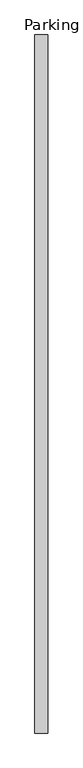
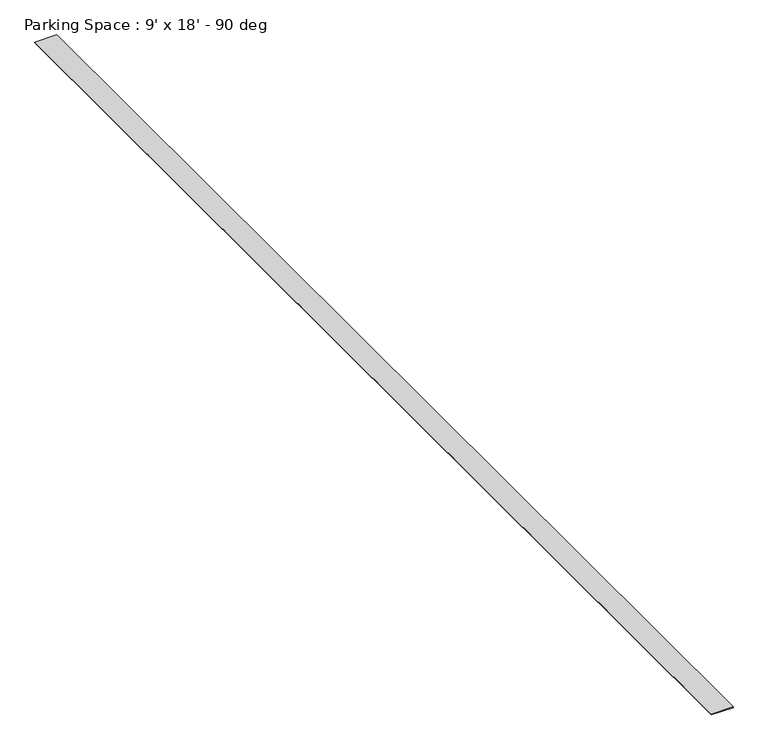
"""IFC4 building model written with IfcOpenShell, lengths in millimetres: proxy geometry, Parking Space : 9' x 18' - 90 deg."""

from ifc_helpers import new_model, si_unit, origin, origin_with_axes, place, context, project, spatial, polyline, outline, extrude, source, transform, mapped, element, save


def parking_space_9_x_18_90_deg_b8b21359(model_context):
    return source(origin(), model_context, "Body", "SweptSolid", [
        extrude(outline(polyline([(-50.8, 0.0), (50.8, 0.0), (50.8, -5486.4), (-50.8, -5486.4), (-50.8, 0.0)])), origin_with_axes(), (0.0, 0.0, 1.0), 3.175),
    ])


if __name__ == "__main__":
    model = new_model("IFC4")
    model_context = context("Model", 3, world=origin())
    ifc_project = project(units=[si_unit("LENGTHUNIT", "METRE", prefix="MILLI")], contexts=[model_context])
    site = spatial("IfcSite", under=ifc_project)
    building = spatial("IfcBuilding", under=site)
    placement = place(None, origin())
    parking_space_9_x_18_90_deg_shape = parking_space_9_x_18_90_deg_b8b21359(model_context)
    element("IfcBuildingElementProxy", 1, Name="Parking Space : 9' x 18' - 90 deg", ObjectType="Parking Space : 9' x 18' - 90 deg", at=placement, inside=building, context=model_context, shape_type="MappedRepresentation", body=[
        mapped(parking_space_9_x_18_90_deg_shape, transform((0.0, 0.0, 0.0), x_axis=(1.0, 0.0, 0.0), y_axis=(0.0, 1.0, 0.0), z_axis=(0.0, 0.0, 1.0))),
    ])
    save(model, "model.ifc")

# Revit data of these elements
# Type "Parking Space : 9' x 18' - 90 deg"
#   Angle = 90.00°
#   Parking Length = 18' - 0"
#   Parking Width = 9' - 0"
#   pl = 18' - 0"
#   pw = 9' - 0"
# Element 1 (IfcBuildingElementProxy, "Parking Space : 9' x 18' - 90 deg")
#   Materials on its faces: "Parking Stripe"
# Materials
#   "Parking Stripe": class "Paint", colour RGB 250 250 91, transparency 0
